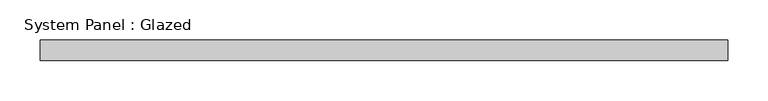
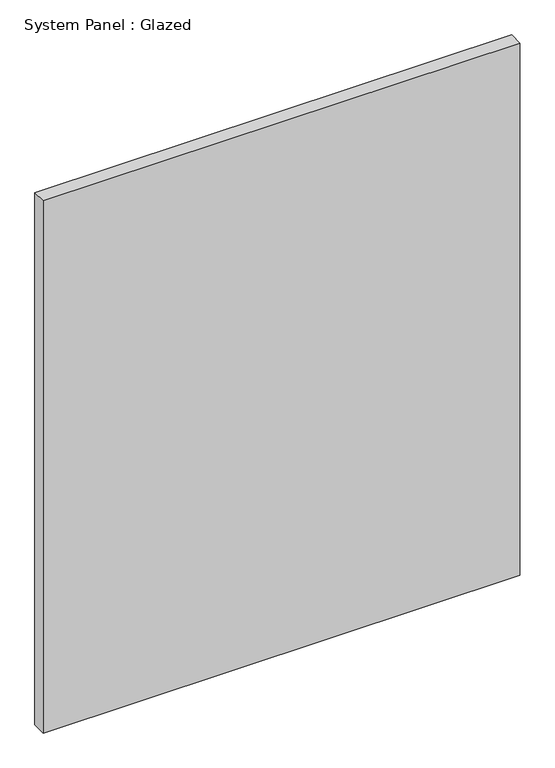
"""IFC4 building model written with IfcOpenShell, lengths in millimetres: plate geometry, System Panel : Glazed."""

from ifc_helpers import new_model, si_unit, origin, origin_with_axes, place, context, project, spatial, polyline, outline, extrude, source, transform, mapped, element, save


def system_panel_glazed_c42ef2fd(model_context):
    return source(origin(), model_context, "Body", "SweptSolid", [
        extrude(outline(polyline([(425.4499999, 19.05), (-425.4499999, 19.05), (-425.4499999, 44.45), (425.4499999, 44.45), (425.4499999, 19.05)])), origin_with_axes(), (0.0, 0.0, 1.0), 1004.3270399),
    ])


if __name__ == "__main__":
    model = new_model("IFC4")
    model_context = context("Model", 3, world=origin())
    ifc_project = project(units=[si_unit("LENGTHUNIT", "METRE", prefix="MILLI")], contexts=[model_context])
    site = spatial("IfcSite", under=ifc_project)
    building = spatial("IfcBuilding", under=site)
    placement = place(None, origin())
    system_panel_glazed_shape = system_panel_glazed_c42ef2fd(model_context)
    element("IfcPlate", 1, ObjectType="System Panel : Glazed", at=placement, inside=building, context=model_context, shape_type="MappedRepresentation", body=[
        mapped(system_panel_glazed_shape, transform((0.0, 0.0, 0.0), x_axis=(1.0, 0.0, 0.0), y_axis=(0.0, 1.0, 0.0), z_axis=(0.0, 0.0, 1.0))),
    ])
    save(model, "model.ifc")

# Revit data of these elements
# Type "System Panel : Glazed"
#   Construction Type Id = "GSP4R"
#   Analytic Construction = "1/8 in Pilkington single glazing"
#   Visual Light Transmittance = 0.9
#   Solar Heat Gain Coefficient = 0.86
#   Heat Transfer Coefficient (U) = 1.18115 BTU/(h·ft²·°F)
#   Define Thermal Properties by = 1
# Element 1 (IfcPlate, "System Panel : Glazed")
#   Materials on its faces: "Glass"
# Materials
#   "Glass": class "Glass", colour RGB 0 128 192, transparency 0.75, Description = "Soda Lime Glass", Cost = 0
